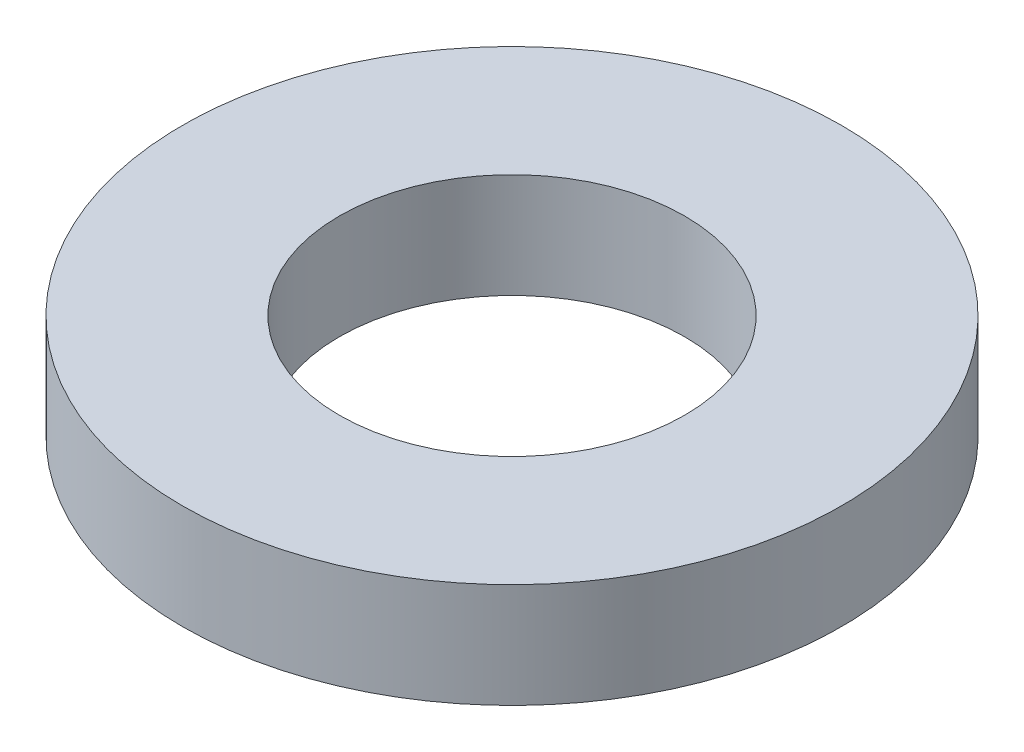
ISO-10303-21;
HEADER;
FILE_DESCRIPTION(('STEP AP214'),'2;1');
FILE_NAME('part.step','',(''),(''),'','','');
FILE_SCHEMA(('AUTOMOTIVE_DESIGN { 1 0 10303 214 1 1 1 1 }'));
ENDSEC;
DATA;
#1=APPLICATION_CONTEXT('core data for automotive mechanical design processes');
#2=APPLICATION_PROTOCOL_DEFINITION('international standard','automotive_design',2000,#1);
#3=PRODUCT_CONTEXT('',#1,'mechanical');
#4=PRODUCT('Part','Part','',(#3));
#5=PRODUCT_RELATED_PRODUCT_CATEGORY('part','',(#4));
#6=PRODUCT_DEFINITION_FORMATION('','',#4);
#7=PRODUCT_DEFINITION_CONTEXT('part definition',#1,'design');
#8=PRODUCT_DEFINITION('design','',#6,#7);
#9=PRODUCT_DEFINITION_SHAPE('','',#8);
#10=(LENGTH_UNIT() NAMED_UNIT(*) SI_UNIT(.MILLI.,.METRE.));
#11=(NAMED_UNIT(*) PLANE_ANGLE_UNIT() SI_UNIT($,.RADIAN.));
#12=(NAMED_UNIT(*) SI_UNIT($,.STERADIAN.) SOLID_ANGLE_UNIT());
#13=UNCERTAINTY_MEASURE_WITH_UNIT(LENGTH_MEASURE(1.E-05),#10,'distance_accuracy_value','');
#14=(GEOMETRIC_REPRESENTATION_CONTEXT(3) GLOBAL_UNCERTAINTY_ASSIGNED_CONTEXT((#13)) GLOBAL_UNIT_ASSIGNED_CONTEXT((#10,
#11,#12)) REPRESENTATION_CONTEXT('',''));
#15=CARTESIAN_POINT('',(0.,0.,0.));
#16=DIRECTION('',(0.,0.,1.));
#17=DIRECTION('',(1.,0.,0.));
#18=AXIS2_PLACEMENT_3D('',#15,#16,#17);
#19=CARTESIAN_POINT('',(0.,5.,0.));
#20=DIRECTION('',(0.,1.,0.));
#21=DIRECTION('',(0.,0.,1.));
#22=AXIS2_PLACEMENT_3D('',#19,#20,#21);
#23=PLANE('',#22);
#24=CARTESIAN_POINT('',(0.,5.,0.));
#25=DIRECTION('',(0.,1.,0.));
#26=DIRECTION('',(0.,0.,1.));
#27=AXIS2_PLACEMENT_3D('',#24,#25,#26);
#28=CIRCLE('',#27,31.5);
#29=CARTESIAN_POINT('',(0.,5.,31.5));
#30=VERTEX_POINT('',#29);
#31=EDGE_CURVE('E10',#30,#30,#28,.T.);
#32=ORIENTED_EDGE('',*,*,#31,.T.);
#33=EDGE_LOOP('',(#32));
#34=FACE_BOUND('',#33,.T.);
#35=CARTESIAN_POINT('',(0.,5.,0.));
#36=DIRECTION('',(0.,1.,0.));
#37=DIRECTION('',(0.,0.,1.));
#38=AXIS2_PLACEMENT_3D('',#35,#36,#37);
#39=CIRCLE('',#38,16.5);
#40=CARTESIAN_POINT('',(0.,5.,16.5));
#41=VERTEX_POINT('',#40);
#42=EDGE_CURVE('E48',#41,#41,#39,.T.);
#43=ORIENTED_EDGE('',*,*,#42,.F.);
#44=EDGE_LOOP('',(#43));
#45=FACE_BOUND('',#44,.T.);
#46=ADVANCED_FACE('F40',(#34,#45),#23,.T.);
#47=CARTESIAN_POINT('',(0.,-5.,0.));
#48=DIRECTION('',(0.,1.,0.));
#49=DIRECTION('',(0.,0.,1.));
#50=AXIS2_PLACEMENT_3D('',#47,#48,#49);
#51=PLANE('',#50);
#52=CARTESIAN_POINT('',(0.,-5.,0.));
#53=DIRECTION('',(0.,1.,0.));
#54=DIRECTION('',(0.,0.,1.));
#55=AXIS2_PLACEMENT_3D('',#52,#53,#54);
#56=CIRCLE('',#55,31.5);
#57=CARTESIAN_POINT('',(0.,-5.,31.5));
#58=VERTEX_POINT('',#57);
#59=EDGE_CURVE('E41',#58,#58,#56,.T.);
#60=ORIENTED_EDGE('',*,*,#59,.F.);
#61=EDGE_LOOP('',(#60));
#62=FACE_BOUND('',#61,.T.);
#63=CARTESIAN_POINT('',(0.,-5.,0.));
#64=DIRECTION('',(0.,1.,0.));
#65=DIRECTION('',(0.,0.,1.));
#66=AXIS2_PLACEMENT_3D('',#63,#64,#65);
#67=CIRCLE('',#66,16.5);
#68=CARTESIAN_POINT('',(0.,-5.,16.5));
#69=VERTEX_POINT('',#68);
#70=EDGE_CURVE('E49',#69,#69,#67,.T.);
#71=ORIENTED_EDGE('',*,*,#70,.T.);
#72=EDGE_LOOP('',(#71));
#73=FACE_BOUND('',#72,.T.);
#74=ADVANCED_FACE('F58',(#62,#73),#51,.F.);
#75=CARTESIAN_POINT('',(0.,5.,0.));
#76=DIRECTION('',(0.,-1.,0.));
#77=DIRECTION('',(0.,0.,-1.));
#78=AXIS2_PLACEMENT_3D('',#75,#76,#77);
#79=CYLINDRICAL_SURFACE('',#78,31.5);
#80=ORIENTED_EDGE('',*,*,#31,.F.);
#81=EDGE_LOOP('',(#80));
#82=FACE_BOUND('',#81,.T.);
#83=ORIENTED_EDGE('',*,*,#59,.T.);
#84=EDGE_LOOP('',(#83));
#85=FACE_BOUND('',#84,.T.);
#86=ADVANCED_FACE('F39',(#82,#85),#79,.T.);
#87=CARTESIAN_POINT('',(0.,5.,0.));
#88=DIRECTION('',(0.,-1.,0.));
#89=DIRECTION('',(0.,0.,-1.));
#90=AXIS2_PLACEMENT_3D('',#87,#88,#89);
#91=CYLINDRICAL_SURFACE('',#90,16.5);
#92=ORIENTED_EDGE('',*,*,#42,.T.);
#93=EDGE_LOOP('',(#92));
#94=FACE_BOUND('',#93,.T.);
#95=ORIENTED_EDGE('',*,*,#70,.F.);
#96=EDGE_LOOP('',(#95));
#97=FACE_BOUND('',#96,.T.);
#98=ADVANCED_FACE('F57',(#94,#97),#91,.F.);
#99=CLOSED_SHELL('',(#46,#74,#86,#98));
#100=MANIFOLD_SOLID_BREP('B2',#99);
#101=ADVANCED_BREP_SHAPE_REPRESENTATION('',(#18,#100),#14);
#102=SHAPE_DEFINITION_REPRESENTATION(#9,#101);
ENDSEC;
END-ISO-10303-21;
